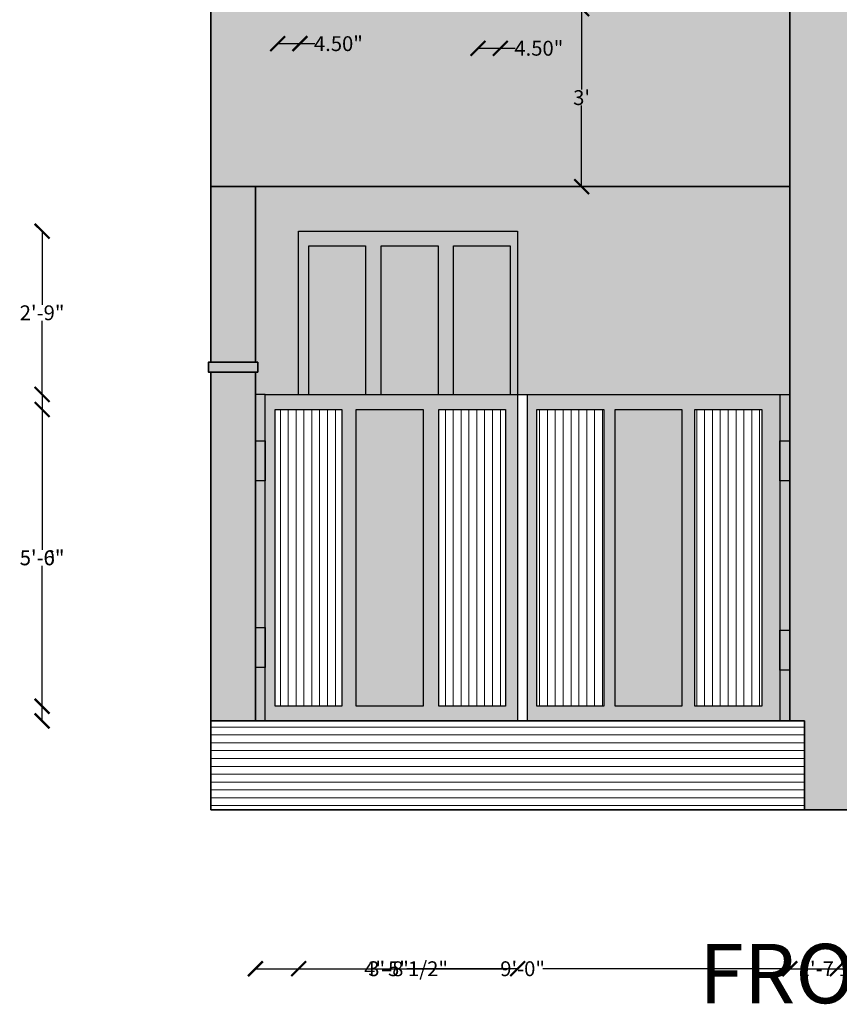
# Model space of a CAD drawing. Units: inches. Extents: x -654 to 390, y -40 to 648.
# Tile 3 of 13: x -40 to 126, y -40 to 159. Entities that reach past the tile are written whole.
import ezdxf

# ---------------------------------------------------------------- set-up
doc = ezdxf.new("R2010")
doc.units = ezdxf.units.IN
doc.header["$PDMODE"] = 3
for name, color, linetype, lineweight in [('A-ANNO-DIMS', 2, 'Continuous', 18), ('A-ANNO-TEXT', 7, 'Continuous', 25), ('A-DOOR', 3, 'Continuous', 25), ('A-ELEV', 7, 'Continuous', 35), ('A-ELEV-FILL', 252, 'Continuous', 13), ('A-ELEV-PATT', 8, 'Continuous', 13), ('A-GLAZ', 4, 'Continuous', 25)]:
    doc.layers.add(name, color=color, linetype=linetype, lineweight=lineweight)
doc.styles.get("Standard").update_dxf_attribs({"font": 'arial.ttf'})
doc.dimstyles.get("Standard").update_dxf_attribs({"dimtxt": 3, "dimasz": 3, "dimexe": 0.18, "dimexo": 0.0625, "dimgap": 0.09, "dimtad": 0, "dimtih": 1, "dimtoh": 1, "dimzin": 0, "dimdsep": 46, "dimlunit": 3, "dimtxsty": 'Standard', "dimblk": 'ARCHTICK', "dimcen": 0.09, "dimse1": 1, "dimse2": 1, "dimadec": 0, "dimazin": 0, "dimtfac": 1, "dimtofl": 0, "dimtmove": 0, "dimatfit": 3, "dimfxl": 1, "dimtolj": 1, "dimtzin": 0, "dimarcsym": 0})

# ---------------------------------------------------------------- blocks, each defined once
blk = doc.blocks.new('_ArchTick')
at = {"color": 0, "linetype": 'ByBlock', "const_width": 0.15}
blk.add_lwpolyline([(-0.5, -0.5), (0.5, 0.5)], dxfattribs=at)
blk = doc.blocks.new('*D24')
at = {"layer": 'A-ANNO-DIMS', "color": 0, "lineweight": -2, "transparency": 16777216}
for p, q in [((73.57, 161.13), (73.57, 144.76)), ((73.57, 125.13), (73.57, 141.51))]:
    blk.add_line(p, q, dxfattribs=at)
at = {"layer": 'Defpoints', "color": 0, "transparency": 16777216}
for p in [(57.15, 161.13), (73.57, 125.13), (73.57, 125.13)]:
    blk.add_point(p, dxfattribs=at)
at = {"layer": 'A-ANNO-DIMS', "color": 0, "lineweight": -2, "transparency": 16777216, "xscale": 3, "yscale": 3, "zscale": 3}
for p, rotation in [((73.57, 161.13), 90), ((73.57, 125.13), 270)]:
    blk.add_blockref('_ArchTick', p, dxfattribs=dict(at, rotation=rotation))
at = {"layer": 'A-ANNO-DIMS', "color": 0, "transparency": 16777216, "insert": (73.57, 143.13), "char_height": 3, "attachment_point": 5}
blk.add_mtext("\\A1;3'", dxfattribs=at)
blk = doc.blocks.new('*D65')
at = {"layer": 'A-ANNO-DIMS', "color": 0, "lineweight": -2, "transparency": 16777216}
for p, q in [((-1.35, 245.3), (12.15, 245.3)), ((12.15, 245.3), (15.15, 245.3))]:
    blk.add_line(p, q, dxfattribs=at)
at = {"layer": 'Defpoints', "color": 0, "transparency": 16777216}
for p in [(12.15, 245.3), (12.15, 161.13), (-1.35, 125.13)]:
    blk.add_point(p, dxfattribs=at)
at = {"layer": 'A-ANNO-DIMS', "color": 0, "lineweight": -2, "transparency": 16777216, "xscale": 3, "yscale": 3, "zscale": 3, "rotation": 180}
blk.add_blockref('_ArchTick', (-1.35, 245.3), dxfattribs=at)
at = {"layer": 'A-ANNO-DIMS', "color": 0, "lineweight": -2, "transparency": 16777216, "xscale": 3, "yscale": 3, "zscale": 3}
blk.add_blockref('_ArchTick', (12.15, 245.3), dxfattribs=at)
at = {"layer": 'A-ANNO-DIMS', "color": 0, "transparency": 16777216, "insert": (22, 245.3), "char_height": 3, "attachment_point": 5}
blk.add_mtext('\\A1;1\'-1.50"', dxfattribs=at)
blk = doc.blocks.new('*D67')
at = {"layer": 'A-ANNO-DIMS', "color": 0, "lineweight": -2, "transparency": 16777216}
for p, q in [((52.65, 153.11), (57.15, 153.11)), ((57.15, 153.11), (60.15, 153.11))]:
    blk.add_line(p, q, dxfattribs=at)
at = {"layer": 'Defpoints', "color": 0, "transparency": 16777216}
for p in [(52.65, 165.63), (57.15, 161.13), (57.15, 153.11)]:
    blk.add_point(p, dxfattribs=at)
at = {"layer": 'A-ANNO-DIMS', "color": 0, "lineweight": -2, "transparency": 16777216, "xscale": 3, "yscale": 3, "zscale": 3, "rotation": 180}
blk.add_blockref('_ArchTick', (52.65, 153.11), dxfattribs=at)
at = {"layer": 'A-ANNO-DIMS', "color": 0, "lineweight": -2, "transparency": 16777216, "xscale": 3, "yscale": 3, "zscale": 3}
blk.add_blockref('_ArchTick', (57.15, 153.11), dxfattribs=at)
at = {"layer": 'A-ANNO-DIMS', "color": 0, "transparency": 16777216, "insert": (64.93, 153.11), "char_height": 3, "attachment_point": 5}
blk.add_mtext('\\A1;4.50"', dxfattribs=at)
blk = doc.blocks.new('*D68')
at = {"layer": 'A-ANNO-DIMS', "color": 0, "lineweight": -2, "transparency": 16777216}
for p, q in [((12.15, 154.04), (16.65, 154.04)), ((16.65, 154.04), (19.65, 154.04))]:
    blk.add_line(p, q, dxfattribs=at)
at = {"layer": 'Defpoints', "color": 0, "transparency": 16777216}
for p in [(16.65, 165.63), (12.15, 161.13), (16.65, 154.04)]:
    blk.add_point(p, dxfattribs=at)
at = {"layer": 'A-ANNO-DIMS', "color": 0, "lineweight": -2, "transparency": 16777216, "xscale": 3, "yscale": 3, "zscale": 3, "rotation": 180}
blk.add_blockref('_ArchTick', (12.15, 154.04), dxfattribs=at)
at = {"layer": 'A-ANNO-DIMS', "color": 0, "lineweight": -2, "transparency": 16777216, "xscale": 3, "yscale": 3, "zscale": 3}
blk.add_blockref('_ArchTick', (16.65, 154.04), dxfattribs=at)
at = {"layer": 'A-ANNO-DIMS', "color": 0, "transparency": 16777216, "insert": (24.43, 154.04), "char_height": 3, "attachment_point": 5}
blk.add_mtext('\\A1;4.50"', dxfattribs=at)
blk = doc.blocks.new('*D77')
at = {"layer": 'A-ANNO-DIMS', "color": 0, "lineweight": -2, "transparency": 16777216}
for p, q in [((7.65, -32.97), (57.57, -32.97)), ((115.65, -32.97), (65.72, -32.97))]:
    blk.add_line(p, q, dxfattribs=at)
at = {"layer": 'Defpoints', "color": 0, "transparency": 16777216}
for p in [(7.65, 17.13), (115.65, 17.13), (115.65, -32.97)]:
    blk.add_point(p, dxfattribs=at)
at = {"layer": 'A-ANNO-DIMS', "color": 0, "lineweight": -2, "transparency": 16777216, "xscale": 3, "yscale": 3, "zscale": 3, "rotation": 180}
blk.add_blockref('_ArchTick', (7.65, -32.97), dxfattribs=at)
at = {"layer": 'A-ANNO-DIMS', "color": 0, "lineweight": -2, "transparency": 16777216, "xscale": 3, "yscale": 3, "zscale": 3}
blk.add_blockref('_ArchTick', (115.65, -32.97), dxfattribs=at)
at = {"layer": 'A-ANNO-DIMS', "color": 0, "transparency": 16777216, "insert": (61.65, -32.97), "char_height": 3, "attachment_point": 5}
blk.add_mtext('\\A1;9\'-0"', dxfattribs=at)
blk = doc.blocks.new('*D78')
at = {"layer": 'A-ANNO-DIMS', "color": 0, "lineweight": -2, "transparency": 16777216}
for p, q in [((-35.45, 83.13), (-35.45, 51.76)), ((-35.45, 17.13), (-35.45, 48.51))]:
    blk.add_line(p, q, dxfattribs=at)
at = {"layer": 'Defpoints', "color": 0, "transparency": 16777216}
for p in [(-35.45, 83.13), (7.65, 83.13), (7.65, 17.13)]:
    blk.add_point(p, dxfattribs=at)
at = {"layer": 'A-ANNO-DIMS', "color": 0, "lineweight": -2, "transparency": 16777216, "xscale": 3, "yscale": 3, "zscale": 3}
for p, rotation in [((-35.45, 83.13), 90), ((-35.45, 17.13), 270)]:
    blk.add_blockref('_ArchTick', p, dxfattribs=dict(at, rotation=rotation))
at = {"layer": 'A-ANNO-DIMS', "color": 0, "transparency": 16777216, "insert": (-35.45, 50.13), "char_height": 3, "attachment_point": 5}
blk.add_mtext('\\A1;5\'-6"', dxfattribs=at)
blk = doc.blocks.new('*D79')
at = {"layer": 'A-ANNO-DIMS', "color": 0, "lineweight": -2, "transparency": 16777216}
for p, q in [((7.65, -32.97), (30.01, -32.97)), ((60.65, -32.97), (38.28, -32.97))]:
    blk.add_line(p, q, dxfattribs=at)
at = {"layer": 'Defpoints', "color": 0, "transparency": 16777216}
for p in [(7.65, 83.13), (60.65, 83.13), (60.65, -32.97)]:
    blk.add_point(p, dxfattribs=at)
at = {"layer": 'A-ANNO-DIMS', "color": 0, "lineweight": -2, "transparency": 16777216, "xscale": 3, "yscale": 3, "zscale": 3, "rotation": 180}
blk.add_blockref('_ArchTick', (7.65, -32.97), dxfattribs=at)
at = {"layer": 'A-ANNO-DIMS', "color": 0, "lineweight": -2, "transparency": 16777216, "xscale": 3, "yscale": 3, "zscale": 3}
blk.add_blockref('_ArchTick', (60.65, -32.97), dxfattribs=at)
at = {"layer": 'A-ANNO-DIMS', "color": 0, "transparency": 16777216, "insert": (34.15, -32.97), "char_height": 3, "attachment_point": 5}
blk.add_mtext('\\A1;4\'-5"', dxfattribs=at)
blk = doc.blocks.new('*D80')
at = {"layer": 'A-ANNO-DIMS', "color": 0, "lineweight": -2, "transparency": 16777216}
for p, q in [((11.65, 643.23), (25.15, 643.23)), ((25.15, 643.23), (28.15, 643.23))]:
    blk.add_line(p, q, dxfattribs=at)
at = {"layer": 'Defpoints', "color": 0, "transparency": 16777216}
for p in [(25.15, 643.23), (11.65, 20.08), (25.15, 20.08)]:
    blk.add_point(p, dxfattribs=at)
at = {"layer": 'A-ANNO-DIMS', "color": 0, "lineweight": -2, "transparency": 16777216, "xscale": 3, "yscale": 3, "zscale": 3, "rotation": 180}
blk.add_blockref('_ArchTick', (11.65, 643.23), dxfattribs=at)
at = {"layer": 'A-ANNO-DIMS', "color": 0, "lineweight": -2, "transparency": 16777216, "xscale": 3, "yscale": 3, "zscale": 3}
blk.add_blockref('_ArchTick', (25.15, 643.23), dxfattribs=at)
at = {"layer": 'A-ANNO-DIMS', "color": 0, "transparency": 16777216, "insert": (35.58, 643.23), "char_height": 3, "attachment_point": 5}
blk.add_mtext('\\A1;1\'-1 1/2"', dxfattribs=at)
blk = doc.blocks.new('*D81')
at = {"layer": 'A-ANNO-DIMS', "color": 0, "lineweight": -2, "transparency": 16777216}
for p, q in [((-35.45, 80.08), (-35.45, 51.7)), ((-35.45, 20.08), (-35.45, 48.46))]:
    blk.add_line(p, q, dxfattribs=at)
at = {"layer": 'Defpoints', "color": 0, "transparency": 16777216}
for p in [(-35.45, 80.08), (11.65, 80.08), (11.65, 20.08)]:
    blk.add_point(p, dxfattribs=at)
at = {"layer": 'A-ANNO-DIMS', "color": 0, "lineweight": -2, "transparency": 16777216, "xscale": 3, "yscale": 3, "zscale": 3}
for p, rotation in [((-35.45, 80.08), 90), ((-35.45, 20.08), 270)]:
    blk.add_blockref('_ArchTick', p, dxfattribs=dict(at, rotation=rotation))
at = {"layer": 'A-ANNO-DIMS', "color": 0, "transparency": 16777216, "insert": (-35.45, 50.08), "char_height": 3, "attachment_point": 5}
blk.add_mtext('\\A1;5\'-0"', dxfattribs=at)
blk = doc.blocks.new('*D82')
at = {"layer": 'A-ANNO-DIMS', "color": 0, "lineweight": -2, "transparency": 16777216}
for p, q in [((16.4, -32.97), (30.95, -32.97)), ((60.65, -32.97), (46.09, -32.97))]:
    blk.add_line(p, q, dxfattribs=at)
at = {"layer": 'Defpoints', "color": 0, "transparency": 16777216}
for p in [(16.4, 116.13), (60.65, 116.13), (60.65, -32.97)]:
    blk.add_point(p, dxfattribs=at)
at = {"layer": 'A-ANNO-DIMS', "color": 0, "lineweight": -2, "transparency": 16777216, "xscale": 3, "yscale": 3, "zscale": 3, "rotation": 180}
blk.add_blockref('_ArchTick', (16.4, -32.97), dxfattribs=at)
at = {"layer": 'A-ANNO-DIMS', "color": 0, "lineweight": -2, "transparency": 16777216, "xscale": 3, "yscale": 3, "zscale": 3}
blk.add_blockref('_ArchTick', (60.65, -32.97), dxfattribs=at)
at = {"layer": 'A-ANNO-DIMS', "color": 0, "transparency": 16777216, "insert": (38.52, -32.97), "char_height": 3, "attachment_point": 5}
blk.add_mtext('\\A1;3\'-8 1/2"', dxfattribs=at)
blk = doc.blocks.new('*D83')
at = {"layer": 'A-ANNO-DIMS', "color": 0, "lineweight": -2, "transparency": 16777216}
for p, q in [((-35.45, 116.13), (-35.45, 101.26)), ((-35.45, 83.13), (-35.45, 98.01))]:
    blk.add_line(p, q, dxfattribs=at)
at = {"layer": 'Defpoints', "color": 0, "transparency": 16777216}
for p in [(-35.45, 116.13), (16.4, 116.13), (16.4, 83.13)]:
    blk.add_point(p, dxfattribs=at)
at = {"layer": 'A-ANNO-DIMS', "color": 0, "lineweight": -2, "transparency": 16777216, "xscale": 3, "yscale": 3, "zscale": 3}
for p, rotation in [((-35.45, 116.13), 90), ((-35.45, 83.13), 270)]:
    blk.add_blockref('_ArchTick', p, dxfattribs=dict(at, rotation=rotation))
at = {"layer": 'A-ANNO-DIMS', "color": 0, "transparency": 16777216, "insert": (-35.45, 99.63), "char_height": 3, "attachment_point": 5}
blk.add_mtext('\\A1;2\'-9"', dxfattribs=at)
blk = doc.blocks.new('*D84')
at = {"layer": 'A-ANNO-DIMS', "color": 0, "lineweight": -2, "transparency": 16777216}
for p, q in [((115.65, -32.97), (118.07, -32.97)), ((135.36, -32.97), (132.94, -32.97))]:
    blk.add_line(p, q, dxfattribs=at)
at = {"layer": 'Defpoints', "color": 0, "transparency": 16777216}
for p in [(115.65, 83.13), (135.36, 71.63), (135.36, -32.97)]:
    blk.add_point(p, dxfattribs=at)
at = {"layer": 'A-ANNO-DIMS', "color": 0, "lineweight": -2, "transparency": 16777216, "xscale": 3, "yscale": 3, "zscale": 3, "rotation": 180}
blk.add_blockref('_ArchTick', (115.65, -32.97), dxfattribs=at)
at = {"layer": 'A-ANNO-DIMS', "color": 0, "lineweight": -2, "transparency": 16777216, "xscale": 3, "yscale": 3, "zscale": 3}
blk.add_blockref('_ArchTick', (135.36, -32.97), dxfattribs=at)
at = {"layer": 'A-ANNO-DIMS', "color": 0, "transparency": 16777216, "insert": (125.5, -32.97), "char_height": 3, "attachment_point": 5}
blk.add_mtext('\\A1;1\'-7 1/2"', dxfattribs=at)
blk = doc.blocks.new('*D92')
at = {"layer": 'A-ANNO-DIMS', "color": 0, "lineweight": -2, "transparency": 16777216}
for p, q in [((115.65, -32.97), (125.23, -32.97)), ((125.23, -32.97), (128.23, -32.97))]:
    blk.add_line(p, q, dxfattribs=at)
at = {"layer": 'Defpoints', "color": 0, "transparency": 16777216}
for p in [(115.65, 305.63), (125.23, 271.79), (125.23, -32.97)]:
    blk.add_point(p, dxfattribs=at)
at = {"layer": 'A-ANNO-DIMS', "color": 0, "lineweight": -2, "transparency": 16777216, "xscale": 3, "yscale": 3, "zscale": 3, "rotation": 180}
blk.add_blockref('_ArchTick', (115.65, -32.97), dxfattribs=at)
at = {"layer": 'A-ANNO-DIMS', "color": 0, "lineweight": -2, "transparency": 16777216, "xscale": 3, "yscale": 3, "zscale": 3}
blk.add_blockref('_ArchTick', (125.23, -32.97), dxfattribs=at)
at = {"layer": 'A-ANNO-DIMS', "color": 0, "transparency": 16777216, "insert": (135.8, -32.97), "char_height": 3, "attachment_point": 5}
blk.add_mtext('\\A1;0\'-9 1/2"', dxfattribs=at)
blk = doc.blocks.new('*D93')
at = {"layer": 'A-ANNO-DIMS', "color": 0, "lineweight": -2, "transparency": 16777216}
for p, q in [((125.23, -32.97), (169.2, -32.97)), ((221.33, -32.97), (177.36, -32.97))]:
    blk.add_line(p, q, dxfattribs=at)
at = {"layer": 'Defpoints', "color": 0, "transparency": 16777216}
for p in [(125.23, 271.79), (221.33, 271.79), (221.33, -32.97)]:
    blk.add_point(p, dxfattribs=at)
at = {"layer": 'A-ANNO-DIMS', "color": 0, "lineweight": -2, "transparency": 16777216, "xscale": 3, "yscale": 3, "zscale": 3, "rotation": 180}
blk.add_blockref('_ArchTick', (125.23, -32.97), dxfattribs=at)
at = {"layer": 'A-ANNO-DIMS', "color": 0, "lineweight": -2, "transparency": 16777216, "xscale": 3, "yscale": 3, "zscale": 3}
blk.add_blockref('_ArchTick', (221.33, -32.97), dxfattribs=at)
at = {"layer": 'A-ANNO-DIMS', "color": 0, "transparency": 16777216, "insert": (173.28, -32.97), "char_height": 3, "attachment_point": 5}
blk.add_mtext('\\A1;8\'-0"', dxfattribs=at)

msp = doc.modelspace()

# ---------------------------------------------------------------- hatches: boundary and pattern name
at = {"layer": 'A-ELEV-FILL'}
h = msp.add_hatch(color=256, dxfattribs=at)
h.dxf.hatch_style = 1
h.paths.add_polyline_path([(115.646, 305.634), (97.646, 305.634), (97.646, 306.634), (98.293, 306.634), (98.293, 315.634), (97.646, 315.634), (97.646, 316.634), (100.646, 316.634), (100.646, 442.634), (-1.354, 442.634), (-1.354, 125.134), (115.646, 125.134)])
h.paths.add_polyline_path([(57.146, 161.134), (12.146, 161.134), (12.146, 413.134), (57.146, 413.134)], flags=16)
h.paths.add_polyline_path([(52.646, 165.634), (16.646, 165.634), (16.646, 408.634), (52.646, 408.634)], flags=0)
h.paths.add_polyline_path([(52.146, 166.134), (17.146, 166.134), (17.146, 408.134), (52.146, 408.134)], flags=0)
h.paths.add_polyline_path([(124.646, 581.134), (-1.354, 581.134), (-1.354, 497.134), (8.646, 497.134), (8.646, 494.634), (12.146, 494.634), (12.146, 546.634), (57.146, 546.634), (57.146, 494.634), (124.646, 494.634)])
h.paths.add_polyline_path([(124.646, 609.134), (-1.354, 609.134), (-1.354, 590.134), (124.646, 590.134)])
h = msp.add_hatch(color=256, dxfattribs=at)
h.dxf.hatch_style = 1
h.paths.add_polyline_path([(161.035, 590.134), (-1.354, 590.134), (-1.354, 581.134), (161.035, 581.134)])
h.paths.add_polyline_path([(346.646, 453.634), (-1.354, 453.634), (-1.354, 444.634), (337.646, 444.634), (337.646, 177.634), (178.742, 177.634), (178.742, 173.134), (176.742, 173.134), (176.742, 177.634), (166.742, 177.634), (166.742, 173.134), (164.742, 173.134), (164.742, 177.634), (154.742, 177.634), (154.742, 173.134), (152.742, 173.134), (152.742, 177.634), (142.742, 177.634), (142.742, 173.134), (140.742, 173.134), (140.742, 177.634), (130.742, 177.634), (130.742, 173.134), (128.742, 173.134), (128.742, 177.634), (115.646, 177.634), (115.646, 168.634), (346.646, 168.634), (346.646, 173.134)])
h.paths.add_polyline_path([(7.646, 87.642), (-1.354, 87.642), (-1.354, 17.134), (7.646, 17.134)])
h.paths.add_polyline_path([(16.396, 116.134), (60.646, 116.134), (60.646, 83.134), (62.646, 83.134), (113.646, 83.134), (115.646, 83.134), (115.646, 125.134), (7.646, 125.134), (7.646, 89.642), (8.146, 89.642), (8.146, 87.642), (7.646, 87.642), (7.646, 83.134), (9.646, 83.134), (16.396, 83.134)])
h = msp.add_hatch(color=256, dxfattribs=at)
h.dxf.hatch_style = 1
h.paths.add_polyline_path([(41.55, 80.08), (28.05, 80.08), (28.05, 20.08), (41.55, 20.08)])
h.paths.add_polyline_path([(93.843, 80.08), (80.343, 80.08), (80.343, 20.08), (93.843, 20.08)])
h.paths.add_polyline_path([(337.646, 442.634), (295.646, 442.634), (295.646, 316.634), (304.646, 316.634), (304.646, 315.634), (303.818, 315.634), (303.818, 306.634), (304.646, 306.634), (304.646, 305.634), (295.646, 305.634), (295.646, 177.634), (337.646, 177.634)])
h.paths.add_polyline_path([(346.646, 495.134), (184.646, 495.134), (184.646, 453.634), (346.646, 453.634)])
h.paths.add_polyline_path([(198.646, 473.634), (198.646, 486.134), (332.646, 486.134), (332.646, 473.634)], flags=16)
h.paths.add_polyline_path([(199.646, 474.634), (199.646, 485.134), (331.646, 485.134), (331.646, 474.634)], flags=0)
h = msp.add_hatch(color=256, dxfattribs=at)
h.dxf.hatch_style = 1
h.paths.add_polyline_path([(138.646, 438.634), (107.646, 438.634), (107.646, 359.634), (138.646, 359.634)])
h.paths.add_polyline_path([(136.646, 436.634), (136.646, 361.634), (109.646, 361.634), (109.646, 436.634)], flags=16)
h.paths.add_polyline_path([(179.877, 410.786), (145.646, 410.786), (145.646, 407.786), (153.285, 407.786), (153.285, 357.634), (145.646, 357.634), (145.646, 355.634), (179.877, 355.634)])
h.paths.add_polyline_path([(178.123, 407.786), (178.123, 357.634), (155.286, 357.634), (155.286, 407.786)], flags=16)
h.paths.add_polyline_path([(291.141, 410.786), (239.871, 410.786), (239.871, 355.634), (241.996, 355.634), (241.996, 407.786), (269.317, 407.786), (269.317, 355.634), (271.318, 355.634), (271.318, 407.786), (289.369, 407.786), (289.369, 355.634), (291.141, 355.634)])
h.paths.add_polyline_path([(128.225, 268.786), (128.742, 268.786), (128.742, 271.786), (125.225, 271.786), (125.225, 216.634), (128.225, 216.634)])
h.paths.add_polyline_path([(140.742, 271.786), (130.742, 271.786), (130.742, 268.786), (140.742, 268.786)])
h.paths.add_polyline_path([(152.742, 271.786), (142.742, 271.786), (142.742, 268.786), (152.742, 268.786)])
h.paths.add_polyline_path([(164.742, 271.786), (154.742, 271.786), (154.742, 268.786), (164.742, 268.786)])
h.paths.add_polyline_path([(176.742, 271.786), (167.328, 271.786), (166.742, 271.786), (166.742, 268.786), (167.328, 268.786), (167.328, 216.634), (169.328, 216.634), (169.328, 268.786), (176.742, 268.786)])
h.paths.add_polyline_path([(221.328, 271.786), (178.742, 271.786), (178.742, 268.786), (184.828, 268.786), (184.828, 216.634), (186.829, 216.634), (186.829, 268.786), (202.329, 268.786), (202.329, 216.634), (204.325, 216.634), (204.325, 268.786), (219.825, 268.786), (219.825, 216.634), (221.328, 216.634)])
h.paths.add_polyline_path([(295.646, 271.786), (244.726, 271.786), (244.726, 216.634), (246.481, 216.634), (246.481, 268.786), (269.317, 268.786), (269.317, 216.634), (271.318, 216.634), (271.318, 268.786), (286.818, 268.786), (286.818, 216.634), (288.814, 216.634), (288.814, 268.786), (295.646, 268.786)])
h.paths.add_polyline_path([(295.646, 216.634), (178.742, 216.634), (178.742, 214.634), (295.646, 214.634)])
h.paths.add_polyline_path([(128.742, 216.634), (123.485, 216.634), (123.485, 214.634), (128.742, 214.634)])
h.paths.add_polyline_path([(140.742, 216.634), (130.742, 216.634), (130.742, 214.634), (140.742, 214.634)])
h.paths.add_polyline_path([(152.742, 216.634), (142.742, 216.634), (142.742, 214.634), (152.742, 214.634)])
h.paths.add_polyline_path([(164.742, 216.634), (154.742, 216.634), (154.742, 214.634), (164.742, 214.634)])
h.paths.add_polyline_path([(176.742, 216.634), (166.742, 216.634), (166.742, 214.634), (176.742, 214.634)])
h.paths.add_polyline_path([(128.742, 192.634), (119.386, 192.634), (119.386, 190.634), (128.742, 190.634)])
h.paths.add_polyline_path([(140.742, 192.634), (130.742, 192.634), (130.742, 190.634), (140.742, 190.634)])
h.paths.add_polyline_path([(152.742, 192.634), (142.742, 192.634), (142.742, 190.634), (152.742, 190.634)])
h.paths.add_polyline_path([(164.742, 192.634), (154.742, 192.634), (154.742, 190.634), (164.742, 190.634)])
h.paths.add_polyline_path([(176.742, 192.634), (166.742, 192.634), (166.742, 190.634), (176.742, 190.634)])
h.paths.add_polyline_path([(295.646, 192.634), (178.742, 192.634), (178.742, 190.634), (295.646, 190.634)])
h.paths.add_polyline_path([(189.362, 137.63), (135.362, 137.63), (135.362, 71.63), (189.362, 71.63)])
h.paths.add_polyline_path([(154.862, 134.63), (170.362, 134.63), (170.362, 74.63), (154.862, 74.63)], flags=16)
h.paths.add_polyline_path([(152.862, 134.63), (152.862, 74.63), (137.362, 74.63), (137.362, 134.63)], flags=16)
h.paths.add_polyline_path([(172.358, 134.63), (187.858, 134.63), (187.858, 74.63), (172.358, 74.63)], flags=16)
h.paths.add_polyline_path([(113.646, 83.134), (62.646, 83.134), (62.646, 17.134), (113.646, 17.134)])
h.paths.add_polyline_path([(96.484, 80.08), (109.984, 80.08), (109.984, 20.08), (96.484, 20.08)], flags=16)
h.paths.add_polyline_path([(93.843, 80.08), (93.843, 20.08), (80.343, 20.08), (80.343, 80.08)], flags=16)
h.paths.add_polyline_path([(78.051, 80.08), (78.051, 20.08), (64.551, 20.08), (64.551, 80.08)], flags=16)
h.paths.add_polyline_path([(60.646, 83.134), (9.646, 83.134), (9.646, 17.134), (60.646, 17.134)])
h.paths.add_polyline_path([(58.197, 80.08), (58.197, 20.08), (44.697, 20.08), (44.697, 80.08)], flags=16)
h.paths.add_polyline_path([(41.55, 80.08), (41.55, 20.08), (28.05, 20.08), (28.05, 80.08)], flags=16)
h.paths.add_polyline_path([(25.146, 80.08), (25.146, 20.08), (11.646, 20.08), (11.646, 80.08)], flags=16)
h.paths.add_polyline_path([(9.646, 83.134), (7.646, 83.134), (7.646, 73.776), (9.646, 73.776)])
h.paths.add_polyline_path([(9.646, 65.663), (7.646, 65.663), (7.646, 36.041), (9.646, 36.041)])
h.paths.add_polyline_path([(9.646, 27.928), (7.646, 27.928), (7.646, 17.134), (9.646, 17.134)])
h.paths.add_polyline_path([(115.646, 83.134), (113.646, 83.134), (113.646, 73.776), (115.646, 73.776)])
h.paths.add_polyline_path([(115.646, 65.663), (113.646, 65.663), (113.646, 35.502), (115.646, 35.502)])
h.paths.add_polyline_path([(115.646, 27.389), (113.646, 27.389), (113.646, 17.134), (115.646, 17.134)])
h.paths.add_polyline_path([(8.146, 89.642), (-1.854, 89.642), (-1.854, 87.642), (8.146, 87.642)])
h.paths.add_polyline_path([(245.646, 156.634), (243.646, 156.634), (243.646, 17.134), (245.646, 17.134)])
h.paths.add_polyline_path([(339.646, 156.634), (337.646, 156.634), (337.646, 17.134), (339.646, 17.134)])
h = msp.add_hatch(color=256, dxfattribs=at)
h.dxf.hatch_style = 1
h.paths.add_polyline_path([(60.646, 116.134), (16.396, 116.134), (16.396, 83.134), (18.431, 83.134), (18.431, 113.134), (29.904, 113.134), (29.904, 83.134), (33.082, 83.134), (33.082, 113.134), (44.556, 113.134), (44.556, 83.134), (47.67, 83.134), (47.67, 113.134), (59.143, 113.134), (59.143, 83.134), (60.646, 83.134)])
h.paths.add_polyline_path([(57.146, 413.134), (12.146, 413.134), (12.146, 161.134), (57.146, 161.134)])
h.paths.add_polyline_path([(52.646, 408.634), (52.646, 165.634), (16.646, 165.634), (16.646, 408.634)], flags=16)
h.paths.add_polyline_path([(52.146, 408.134), (52.146, 166.134), (17.146, 166.134), (17.146, 408.134)], flags=0)
h = msp.add_hatch(color=256, dxfattribs=at)
h.dxf.hatch_style = 1
h.paths.add_polyline_path([(243.646, 156.634), (243.146, 156.634), (243.146, 166.634), (340.146, 166.634), (340.146, 156.634), (339.646, 156.634), (339.646, 35.134), (346.646, 35.134), (346.646, 168.634), (115.646, 168.634), (115.646, 17.134), (118.646, 17.134), (118.646, -0.866), (226.646, -0.866), (226.646, 17.134), (243.646, 17.134)])
h.paths.add_polyline_path([(189.362, 71.63), (135.362, 71.63), (135.362, 137.63), (189.362, 137.63)], flags=16)
h.paths.add_polyline_path([(187.858, 74.63), (172.358, 74.63), (172.358, 134.63), (187.858, 134.63)], flags=0)
h.paths.add_polyline_path([(170.362, 74.63), (154.862, 74.63), (154.862, 134.63), (170.362, 134.63)], flags=0)
h.paths.add_polyline_path([(152.862, 74.63), (137.362, 74.63), (137.362, 134.63), (152.862, 134.63)], flags=0)
h.paths.add_polyline_path([(346.646, 35.134), (339.646, 35.134), (339.646, 17.134), (346.646, 17.134)], flags=17)
h = msp.add_hatch(color=256, dxfattribs=at)
h.dxf.hatch_style = 1
h.paths.add_polyline_path([(7.646, 125.134), (-1.354, 125.134), (-1.354, 89.642), (7.646, 89.642)])
h = msp.add_hatch(color=256, dxfattribs=at)
h.dxf.hatch_style = 1
h.paths.add_polyline_path([(9.646, 73.776), (7.646, 73.776), (7.646, 65.663), (9.646, 65.663)])
h.paths.add_polyline_path([(115.646, 73.776), (113.646, 73.776), (113.646, 65.663), (115.646, 65.663)])
h.paths.add_polyline_path([(9.646, 36.041), (7.646, 36.041), (7.646, 27.928), (9.646, 27.928)])
h.paths.add_polyline_path([(115.646, 35.502), (113.646, 35.502), (113.646, 27.389), (115.646, 27.389)])
at = {"layer": 'A-ELEV-PATT'}
h = msp.add_hatch(dxfattribs=at)
h.set_pattern_fill('GOST_GLASS', color=256)
h.paths.add_polyline_path([(34.168, 540.134), (18.646, 540.134), (18.646, 494.634), (34.168, 494.634)])
h.paths.add_polyline_path([(50.651, 540.134), (35.875, 540.134), (35.875, 494.634), (50.651, 494.634)])
h.paths.add_polyline_path([(23.368, 492.634), (18.646, 492.634), (18.646, 482.634), (23.368, 482.634)])
h.paths.add_polyline_path([(30.384, 492.634), (24.368, 492.634), (24.368, 482.634), (30.384, 482.634)])
h.paths.add_polyline_path([(34.168, 492.634), (31.384, 492.634), (31.384, 482.634), (34.168, 482.634)])
h.paths.add_polyline_path([(44.416, 492.634), (38.4, 492.634), (38.4, 482.634), (44.416, 482.634)])
h.paths.add_polyline_path([(50.651, 492.634), (45.416, 492.634), (45.416, 482.634), (50.651, 482.634)])
h.paths.add_polyline_path([(37.4, 492.634), (35.875, 492.634), (35.875, 482.634), (37.4, 482.634)])
h.paths.add_polyline_path([(52.146, 408.134), (17.146, 408.134), (17.146, 360.234), (52.146, 360.234)])
h.paths.add_polyline_path([(52.146, 359.234), (17.146, 359.234), (17.146, 311.834), (52.146, 311.834)])
h.paths.add_polyline_path([(52.146, 310.834), (17.146, 310.834), (17.146, 263.434), (52.146, 263.434)])
h.paths.add_polyline_path([(52.146, 262.434), (17.146, 262.434), (17.146, 215.034), (52.146, 215.034)])
h.paths.add_polyline_path([(52.146, 214.034), (17.146, 214.034), (17.146, 166.134), (52.146, 166.134)])
h.paths.add_polyline_path([(44.556, 113.134), (33.082, 113.134), (33.082, 83.134), (44.556, 83.134)])
h.paths.add_polyline_path([(29.904, 113.134), (18.431, 113.134), (18.431, 83.134), (29.904, 83.134)])
h.paths.add_polyline_path([(59.143, 113.134), (47.67, 113.134), (47.67, 83.134), (59.143, 83.134)])
h.paths.add_polyline_path([(152.862, 134.63), (137.362, 134.63), (137.362, 74.63), (152.862, 74.63)])
h.paths.add_polyline_path([(170.362, 134.63), (154.862, 134.63), (154.862, 74.63), (170.362, 74.63)])
h.paths.add_polyline_path([(187.858, 134.63), (172.358, 134.63), (172.358, 74.63), (187.858, 74.63)])
h = msp.add_hatch(dxfattribs=at)
h.set_pattern_fill('LINE', color=256, scale=0.5, angle=90)
h.paths.add_polyline_path([(25.146, 80.08), (11.646, 80.08), (11.646, 20.08), (25.146, 20.08)])
h.paths.add_polyline_path([(58.197, 80.08), (44.697, 80.08), (44.697, 20.08), (58.197, 20.08)])
h.paths.add_polyline_path([(78.051, 80.08), (64.551, 80.08), (64.551, 20.08), (78.051, 20.08)])
h.paths.add_polyline_path([(109.984, 80.08), (96.484, 80.08), (96.484, 20.08), (109.984, 20.08)])
h = msp.add_hatch(dxfattribs=at)
h.set_pattern_fill('LINE', color=256, scale=0.5)
h.paths.add_polyline_path([(118.646, 17.134), (-1.354, 17.134), (-1.354, -0.866), (118.646, -0.866)])

# ---------------------------------------------------------------- linework, layer by layer
at = {"layer": 'A-DOOR'}
for p, q in [((9.646, 83.134), (7.646, 83.134)), ((60.646, 83.134), (62.646, 83.134)), ((113.646, 83.134), (115.646, 83.134)), ((60.646, 17.134), (62.646, 17.134))]:
    msp.add_line(p, q, dxfattribs=at)
for points in [[(9.646, 83.134), (60.646, 83.134), (60.646, 17.134), (9.646, 17.134)], [(62.646, 83.134), (113.646, 83.134), (113.646, 17.134), (62.646, 17.134)], [(11.646, 80.08), (25.146, 80.08), (25.146, 20.08), (11.646, 20.08)], [(28.05, 80.08), (41.55, 80.08), (41.55, 20.08), (28.05, 20.08)], [(44.697, 80.08), (58.197, 80.08), (58.197, 20.08), (44.697, 20.08)], [(64.551, 80.08), (78.051, 80.08), (78.051, 20.08), (64.551, 20.08)], [(80.343, 80.08), (93.843, 80.08), (93.843, 20.08), (80.343, 20.08)], [(96.484, 80.08), (109.984, 80.08), (109.984, 20.08), (96.484, 20.08)], [(7.646, 73.776), (9.646, 73.776), (9.646, 65.663), (7.646, 65.663)], [(113.646, 73.776), (115.646, 73.776), (115.646, 65.663), (113.646, 65.663)], [(7.646, 36.041), (9.646, 36.041), (9.646, 27.928), (7.646, 27.928)], [(113.646, 35.502), (115.646, 35.502), (115.646, 27.389), (113.646, 27.389)]]:
    msp.add_lwpolyline(points, close=True, dxfattribs=at)
at = {"layer": 'A-ELEV'}
for p, q in [((-1.354, 89.642), (-1.354, 495.134)), ((115.646, 17.134), (115.646, 305.634)), ((-1.354, 125.134), (115.646, 125.134)), ((-1.354, 125.134), (-1.354, 89.642)), ((7.646, 125.134), (7.646, 89.642)), ((115.646, 125.134), (115.646, 17.134)), ((-1.354, -0.866), (-1.354, 87.642)), ((-1.354, 87.642), (-1.354, 17.134)), ((7.646, 87.642), (7.646, 17.134)), ((-1.354, 17.134), (118.646, 17.134)), ((118.646, 17.134), (-1.354, 17.134)), ((118.646, 17.134), (118.646, -0.866)), ((-1.354, -0.866), (346.646, -0.866))]:
    msp.add_line(p, q, dxfattribs=at)
msp.add_lwpolyline([(8.146, 87.642), (-1.854, 87.642), (-1.854, 89.642), (8.146, 89.642)], close=True, dxfattribs=at)
at = {"layer": 'A-GLAZ'}
for points in [[(16.396, 83.134), (16.396, 116.134), (60.646, 116.134), (60.646, 83.134)], [(18.431, 83.134), (18.431, 113.134), (29.904, 113.134), (29.904, 83.134)], [(33.082, 83.134), (33.082, 113.134), (44.556, 113.134), (44.556, 83.134)], [(47.67, 83.134), (47.67, 113.134), (59.143, 113.134), (59.143, 83.134)]]:
    msp.add_lwpolyline(points, dxfattribs=at)

# ---------------------------------------------------------------- texts
at = {"layer": 'A-ANNO-TEXT', "insert": (97.321, -7.947), "char_height": 12, "attachment_point": 1}
msp.add_mtext_dynamic_manual_height_columns('\\PFRONT ELEVATION', width=187.36466, gutter_width=12.5, heights=[0], dxfattribs=at)

# ---------------------------------------------------------------- dimensions: what is measured, and where the dimension line sits
at = {"layer": 'A-ANNO-DIMS'}
for base, p1, p2, override, picture, middle in [((25.146, 643.234), (11.646, 20.08), (25.146, 20.08), {"dimdec": 1, "dimlfac": 1, "dimrnd": 0, "dimzin": 1, "dimdsep": 46, "dimlunit": 4, "dimfrac": 2}, '*D80', (35.578, 643.234)), ((125.225, -32.966), (115.646, 305.634), (125.225, 271.786), {"dimdec": 1, "dimlfac": 1, "dimrnd": 0, "dimzin": 1, "dimdsep": 46, "dimlunit": 4, "dimfrac": 2}, '*D92', (135.798, -32.966)), ((221.328, -32.966), (125.225, 271.786), (221.328, 271.786), {"dimdec": 1, "dimlfac": 1, "dimrnd": 0, "dimzin": 1, "dimdsep": 46, "dimlunit": 4, "dimfrac": 2}, '*D93', (173.277, -32.966)), ((12.146, 245.302), (-1.354, 125.134), (12.146, 161.134), {"dimclrd": 0, "dimclre": 0, "dimclrt": 0}, '*D65', (21.996, 245.302)), ((16.646, 154.036), (12.146, 161.134), (16.646, 165.634), {"dimclrd": 0, "dimclre": 0, "dimclrt": 0}, '*D68', (24.434, 154.036)), ((57.146, 153.11), (52.646, 165.634), (57.146, 161.134), {"dimclrd": 0, "dimclre": 0, "dimclrt": 0}, '*D67', (64.934, 153.11)), ((60.646381, -32.966384), (16.396381, 116.133616), (60.646381, 116.133616), {"dimdec": 1, "dimlfac": 1, "dimrnd": 0, "dimzin": 1, "dimdsep": 46, "dimlunit": 4, "dimfrac": 2}, '*D82', (38.521381, -32.966384)), ((60.646, -32.966), (7.646, 83.134), (60.646, 83.134), {"dimdec": 1, "dimlfac": 1, "dimrnd": 0, "dimzin": 1, "dimdsep": 46, "dimlunit": 4, "dimfrac": 2}, '*D79', (34.146, -32.966)), ((135.362, -32.966), (115.646, 83.134), (135.362, 71.63), {"dimdec": 1, "dimlfac": 1, "dimrnd": 0, "dimzin": 1, "dimdsep": 46, "dimlunit": 4, "dimfrac": 2}, '*D84', (125.504, -32.966)), ((115.646, -32.966), (7.646, 17.134), (115.646, 17.134), {"dimdec": 1, "dimlfac": 1, "dimrnd": 0, "dimzin": 1, "dimdsep": 46, "dimlunit": 4, "dimfrac": 2}, '*D77', (61.646, -32.966))]:
    dim = msp.add_linear_dim(base=base, p1=p1, p2=p2, dimstyle='Standard', override=override, dxfattribs=at)
    dim.commit()
    dim.dimension.update_dxf_attribs({"geometry": picture, "text_midpoint": middle})
for base, p1, p2, override, picture, middle in [((73.566, 125.134), (57.146, 161.134), (73.566, 125.134), {"dimclrd": 0, "dimclre": 0, "dimclrt": 0, "dimtmove": 1}, '*D24', (73.566, 143.134)), ((-35.454, 116.134), (16.396, 83.134), (16.396, 116.134), {"dimdec": 1, "dimlfac": 1, "dimrnd": 0, "dimzin": 1, "dimdsep": 46, "dimlunit": 4, "dimfrac": 2}, '*D83', (-35.454, 99.634)), ((-35.454, 83.134), (7.646, 17.134), (7.646, 83.134), {"dimdec": 1, "dimlfac": 1, "dimrnd": 0, "dimzin": 1, "dimdsep": 46, "dimlunit": 4, "dimfrac": 2}, '*D78', (-35.454, 50.134)), ((-35.454, 80.08), (11.646, 20.08), (11.646, 80.08), {"dimdec": 1, "dimlfac": 1, "dimrnd": 0, "dimzin": 1, "dimdsep": 46, "dimlunit": 4, "dimfrac": 2}, '*D81', (-35.454, 50.08))]:
    dim = msp.add_linear_dim(base=base, p1=p1, p2=p2, angle=90, dimstyle='Standard', override=override, dxfattribs=at)
    dim.commit()
    dim.dimension.update_dxf_attribs({"geometry": picture, "text_midpoint": middle})

doc.saveas('drawing.dxf')
